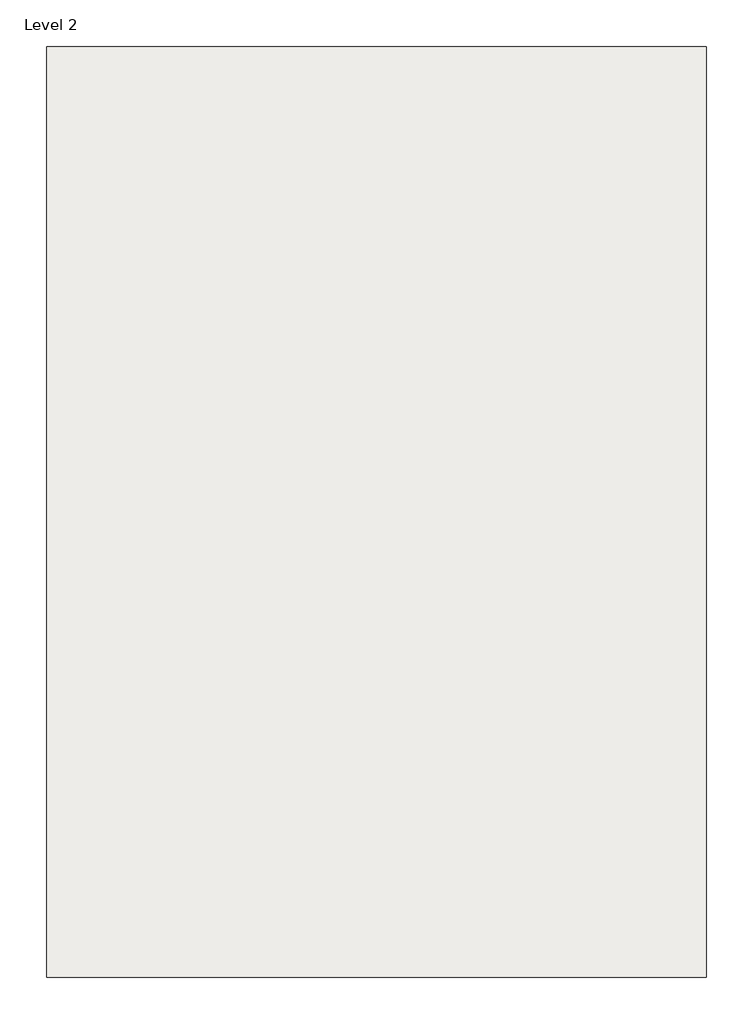
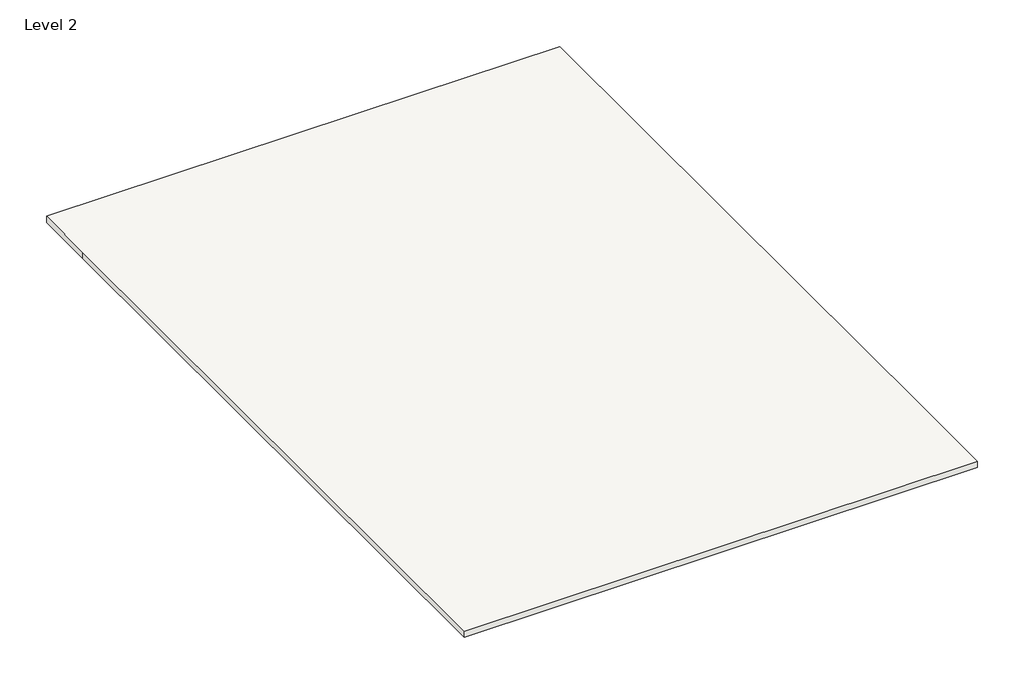
# One storey, incomplete: 1 roof.
"""IFC4 building model written with IfcOpenShell, lengths in millimetres."""

from ifc_helpers import new_model, si_unit, frame, origin, place, context, project, spatial, polyline, outline, extrude, element, save

model = new_model("IFC4")

# Units and contexts
model_context = context("Model", 3, world=origin())
ifc_project = project(units=[si_unit("LENGTHUNIT", "METRE", prefix="MILLI")], contexts=[model_context])

# Site, building, storey
site = spatial("IfcSite", under=ifc_project)
building = spatial("IfcBuilding", under=site)
storey = spatial("IfcBuildingStorey", under=building, Name="Level 2", Elevation=3048.0)

# Roof
placement = place(None, origin())
element("IfcRoof", 1, ObjectType="Generic - 12\"", at=placement, inside=storey, context=model_context, shape_type="SweptSolid", body=[
    extrude(outline(polyline([(9804.4, 28956.0), (13081.0, 28956.0), (13081.0, 19354.8), (13081.0, 14528.8), (13081.0, 12293.6), (1270.0, 12293.6), (1270.0, 27508.2), (1270.0, 28956.0), (9804.4, 28956.0)])), frame((0.0, 0.0, 3048.0), z_axis=(0.0, 0.0, 1.0), x_axis=(1.0, 0.0, 0.0)), (0.0, 0.0, 1.0), 152.4),
])

save(model, "model.ifc")

# Revit data of these elements
# Type "Generic - 12\""
#   Assembly Code = "B1020"
#   Layers, outside or top first: 0' - 6" no material (function 1)
# Element 1 (IfcRoof, "Generic - 12\"")
#   built-in parameter 1001705 = 10.5 (stored number, unit not read)
#   built-in parameter 1001710 = 33615
#   Phase Created = New Construction
#   Materials on its faces: "Default Roof"
# Materials
#   "Default Roof": colour RGB 88 101 114, transparency 0, Cost = 0
